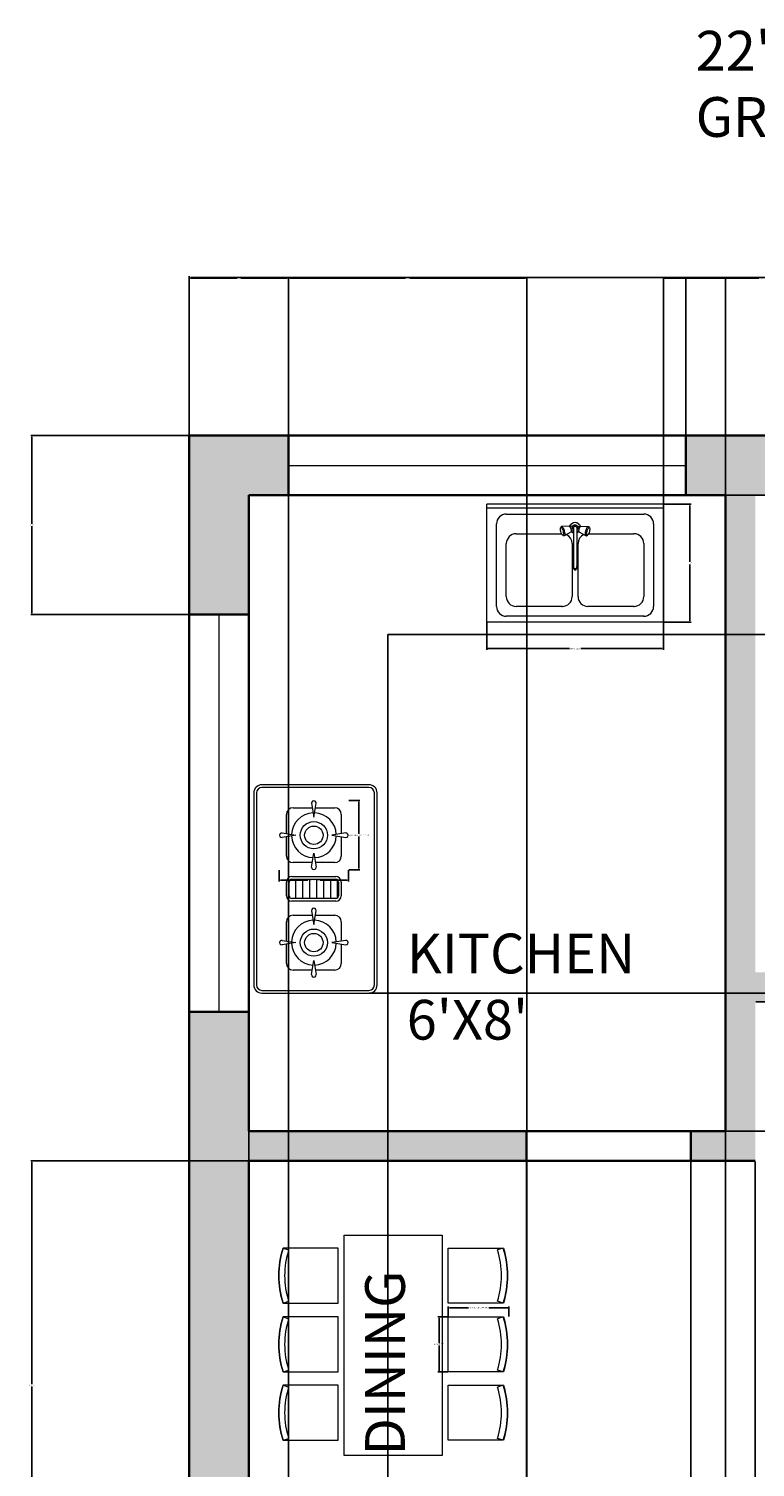
# Model space of a CAD drawing. Units: inches. Extents: x 10 to 332, y -471 to 73.
# Tile 4 of 5: x 10 to 120, y -144 to 73. Entities that reach past the tile are written whole.
import ezdxf

# ---------------------------------------------------------------- set-up
doc = ezdxf.new("R2010")
doc.units = ezdxf.units.IN
doc.header["$MEASUREMENT"] = 0
for name, color, linetype, lineweight in [('A-ANNO-DIMS', 2, 'Continuous', 18), ('A-ANNO-TEXT', 7, 'Continuous', 25), ('A-AREA-IDEN', 7, 'Continuous', 18), ('A-EQPM', 8, 'Continuous', 18), ('A-EQPM-PATT', 8, 'Continuous', 13), ('A-FLOR-CASE', 9, 'Continuous', 25), ('A-FLOR-FIXT', 9, 'Continuous', 18), ('A-FURN', 9, 'Continuous', 18), ('A-GLAZ', 4, 'Continuous', 18), ('A-WALL', 7, 'Continuous', 35), ('A-WALL-PATT', 8, 'Continuous', 13)]:
    doc.layers.add(name, color=color, linetype=linetype, lineweight=lineweight)
doc.styles.get("Standard").update_dxf_attribs({"font": 'arial.ttf'})
doc.dimstyles.get("Standard").update_dxf_attribs({"dimtxt": 0.18, "dimasz": 0.18, "dimexe": 0.18, "dimexo": 0.0625, "dimgap": 0.09, "dimtad": 0, "dimtih": 1, "dimtoh": 1, "dimdec": 0, "dimzin": 0, "dimdsep": 46, "dimlunit": 3, "dimtxsty": 'Standard', "dimcen": 0.09, "dimadec": 0, "dimazin": 0, "dimtfac": 1, "dimtdec": 0, "dimtofl": 0, "dimtmove": 0, "dimatfit": 3, "dimfxl": 1, "dimtolj": 1, "dimtzin": 0, "dimarcsym": 0})

# ---------------------------------------------------------------- blocks, each defined once
blk = doc.blocks.new('М07 600х900')
for p, q in [((0, 600), (-900, 600)), ((-900, 0), (-900, 600)), ((-900, 0), (-900, 600)), ((0, 0), (0, 600)), ((0, 0), (0, 600)), ((0, 580), (-900, 580)), ((-800, 550), (-100, 550)), ((-850, 80), (-850, 500)), ((-750, 450), (-519.1, 450)), ((-524.9, 472.1), (-524.8, 476.7)), ((-524.3, 466.5), (-524.9, 472.1)), ((-524.8, 476.7), (-523.8, 479.9)), ((-523, 460.4), (-524.3, 466.5)), ((-520.9, 485.6), (-523.8, 479.9)), ((-523.8, 479.9), (-522.2, 481.3)), ((-521.1, 454.5), (-523, 460.4)), ((-522.2, 481.3), (-520.1, 480.9)), ((-518.8, 449.4), (-521.1, 454.5)), ((-520.9, 485.6), (-518.9, 487.4)), ((-520.1, 480.9), (-517.7, 478.6)), ((-479.6, 487.6), (-518.9, 487.4)), ((-518.9, 487.4), (-516.3, 486.8)), ((-516.4, 445.5), (-518.8, 449.4)), ((-517.7, 478.6), (-515.3, 474.7)), ((-514, 443.2), (-516.4, 445.5)), ((-516.3, 486.8), (-513.3, 484)), ((-515.3, 474.7), (-513, 469.5)), ((-508.6, 439.7), (-514, 443.2)), ((-511.9, 442.7), (-514, 443.2)), ((-513.3, 484), (-510.2, 479.1)), ((-513, 469.5), (-511.1, 463.6)), ((-510.3, 444.2), (-511.9, 442.7)), ((-511.1, 463.6), (-509.8, 457.6)), ((-509.4, 447.3), (-510.3, 444.2)), ((-510.2, 479.1), (-507.4, 472.6)), ((-509.8, 457.6), (-509.2, 452)), ((-509.2, 452), (-509.4, 447.3)), ((-506, 439.1), (-508.6, 439.7)), ((-507.4, 472.6), (-505, 465.3)), ((-471.8, 458.6), (-506, 439.1)), ((-504, 440.9), (-506, 439.1)), ((-505, 465.3), (-503.4, 457.7)), ((-502.8, 444.9), (-504, 440.9)), ((-503.4, 457.7), (-502.6, 450.7)), ((-502.6, 450.7), (-502.8, 444.9)), ((-479.6, 487.6), (-478, 487.3)), ((-478, 487.3), (-476.2, 485.5)), ((-477, 486.3), (-476.6, 488.7)), ((-476.6, 488.7), (-472.7, 496.5)), ((-461.4, 489.4), (-476.2, 485.4)), ((-476.2, 485.5), (-474.4, 482.6)), ((-474.4, 482.6), (-472.7, 478.7)), ((-472.7, 496.5), (-466.5, 502.7)), ((-472.7, 478.7), (-471.2, 474.3)), ((-470.6, 459.7), (-471.8, 458.6)), ((-471.2, 474.3), (-470.3, 469.8)), ((-469.9, 462.1), (-470.6, 459.7)), ((-470.3, 469.8), (-469.8, 465.6)), ((-466.5, 457.3), (-470.2, 461.1)), ((-469.8, 465.6), (-469.9, 462.1)), ((-458.5, 465.3), (-469.9, 462.2)), ((-466.5, 502.7), (-458.7, 506.6)), ((-458.7, 453.4), (-466.5, 457.3)), ((-465, 480), (-462.1, 488.8)), ((-462.1, 471.2), (-465, 480)), ((-462.1, 488.8), (-454.6, 494.3)), ((-458.5, 468.5), (-462.1, 471.2)), ((-458.7, 506.6), (-450, 508)), ((-458.5, 453.3), (-458.7, 453.4)), ((-458.5, 480), (-456.9, 485)), ((-458.5, 480), (-458.5, 279.9)), ((-456.9, 485), (-452.6, 488.1)), ((-454.6, 494.3), (-445.4, 494.3)), ((-452.6, 488.1), (-447.4, 488.1)), ((-450, 508), (-441.3, 506.6)), ((-447.4, 488.1), (-443.1, 485)), ((-445.4, 494.3), (-437.9, 488.8)), ((-443.1, 485), (-441.5, 480)), ((-441.5, 480), (-441.5, 279.9)), ((-437.9, 471.2), (-441.5, 468.5)), ((-441.5, 465.3), (-430.1, 462.2)), ((-441.3, 453.4), (-441.5, 453.3)), ((-441.3, 506.6), (-433.5, 502.7)), ((-433.5, 457.3), (-441.3, 453.4)), ((-438.6, 489.4), (-423.8, 485.4)), ((-437.9, 488.8), (-435, 480)), ((-435, 480), (-437.9, 471.2)), ((-433.5, 502.7), (-427.3, 496.5)), ((-429.8, 461.1), (-433.5, 457.3)), ((-430.2, 465.6), (-429.7, 469.8)), ((-430.1, 462.1), (-430.2, 465.6)), ((-429.4, 459.7), (-430.1, 462.1)), ((-429.7, 469.8), (-428.8, 474.3)), ((-428.2, 458.6), (-429.4, 459.7)), ((-428.8, 474.3), (-427.3, 478.7)), ((-428.2, 458.6), (-394, 439.1)), ((-427.3, 496.5), (-423.4, 488.7)), ((-427.3, 478.7), (-425.6, 482.6)), ((-425.6, 482.6), (-423.8, 485.5)), ((-423.8, 485.5), (-422, 487.3)), ((-423.4, 488.7), (-423, 486.3)), ((-422, 487.3), (-420.4, 487.6)), ((-420.4, 487.6), (-381.1, 487.4)), ((-397.4, 450.7), (-396.6, 457.7)), ((-397.2, 444.9), (-397.4, 450.7)), ((-396, 440.9), (-397.2, 444.9)), ((-396.6, 457.7), (-395, 465.3)), ((-394, 439.1), (-396, 440.9)), ((-395, 465.3), (-392.6, 472.6)), ((-391.4, 439.7), (-394, 439.1)), ((-392.6, 472.6), (-389.8, 479.1)), ((-391.4, 439.7), (-386, 443.2)), ((-390.8, 452), (-390.2, 457.6)), ((-390.6, 447.3), (-390.8, 452)), ((-389.7, 444.2), (-390.6, 447.3)), ((-390.2, 457.6), (-388.9, 463.6)), ((-389.8, 479.1), (-386.7, 484)), ((-388.1, 442.7), (-389.7, 444.2)), ((-388.9, 463.6), (-387, 469.5)), ((-386, 443.2), (-388.1, 442.7)), ((-387, 469.5), (-384.7, 474.7)), ((-386.7, 484), (-383.7, 486.8)), ((-383.6, 445.5), (-386, 443.2)), ((-384.7, 474.7), (-382.3, 478.6)), ((-383.7, 486.8), (-381.1, 487.4)), ((-381.2, 449.4), (-383.6, 445.5)), ((-382.3, 478.6), (-379.9, 480.9)), ((-378.9, 454.5), (-381.2, 449.4)), ((-381.1, 487.4), (-379.1, 485.6)), ((-380.9, 450), (-150, 450)), ((-379.9, 480.9), (-377.8, 481.3)), ((-379.1, 485.6), (-376.2, 479.9)), ((-377, 460.4), (-378.9, 454.5)), ((-377.8, 481.3), (-376.2, 479.9)), ((-375.7, 466.5), (-377, 460.4)), ((-376.2, 479.9), (-375.2, 476.7)), ((-375.1, 472.1), (-375.7, 466.5)), ((-375.2, 476.7), (-375.1, 472.1)), ((-50, 500), (-50, 80)), ((-800, 130), (-800, 400)), ((-465, 400), (-465, 130)), ((-435, 130), (-435, 400)), ((-100, 400), (-100, 130)), ((-458.5, 285.6), (-460.5, 279.9)), ((-460.5, 279.9), (-458.5, 274.2)), ((-458.5, 279.9), (-456.9, 275.3)), ((-458.5, 274.2), (-456.9, 269.8)), ((-458.5, 274.2), (-453.2, 270.6)), ((-456.9, 275.3), (-452.6, 272.4)), ((-456.9, 269.8), (-452.6, 266.9)), ((-453.2, 270.6), (-446.8, 270.6)), ((-452.6, 272.4), (-447.4, 272.4)), ((-452.6, 266.9), (-447.4, 266.9)), ((-447.4, 272.4), (-443.1, 275.3)), ((-447.4, 266.9), (-443.1, 269.8)), ((-446.8, 270.6), (-441.5, 274.2)), ((-443.1, 275.3), (-441.5, 279.9)), ((-441.5, 274.2), (-443.1, 269.8)), ((-439.5, 279.9), (-441.5, 285.6)), ((-441.5, 274.2), (-439.5, 279.9)), ((-515, 80), (-750, 80)), ((-150, 80), (-385, 80)), ((0, 0), (-900, 0)), ((-100, 30), (-800, 30))]:
    blk.add_line(p, q)
for centre, start, end in [((-800, 500), 90, 180), ((-100, 500), 0, 90), ((-750, 400), 90, 180), ((-515, 400), 0, 65.88741), ((-385, 400), 114.11259, 180), ((-150, 400), 0, 90), ((-800, 80), 180, 270), ((-750, 130), 180, 270), ((-515, 130), 270, 0), ((-385, 130), 180, 270), ((-150, 130), 270, 0), ((-100, 80), 270, 0)]:
    blk.add_arc(centre, 50, start, end)
for p in [(-515, 80), (-150, 80), (-100, 30)]:
    blk.add_point(p)
blk = doc.blocks.new('*D2')
at = {"layer": 'A-ANNO-DIMS', "color": 0, "lineweight": -2, "transparency": 16777216}
for p, q in [((34.37, 12.05), (34.37, 36.05)), ((34.55, 35.87), (157.42, 35.87)), ((301.19, 35.87), (178.31, 35.87)), ((301.37, 12.05), (301.37, 36.05))]:
    blk.add_line(p, q, dxfattribs=at)
at = {"layer": 'A-ANNO-DIMS', "color": 0, "transparency": 16777216}
for points in [[(34.55, 35.9), (34.55, 35.84), (34.37, 35.87)], [(301.19, 35.9), (301.19, 35.84), (301.37, 35.87)]]:
    blk.add_solid(points, dxfattribs=at)
at = {"layer": 'Defpoints', "color": 0, "transparency": 16777216}
for p in [(301.37, 35.87), (34.37, 11.99), (301.37, 11.99)]:
    blk.add_point(p, dxfattribs=at)
at = {"layer": 'A-ANNO-DIMS', "color": 0, "transparency": 16777216, "insert": (167.87, 35.87), "char_height": 6, "attachment_point": 5}
blk.add_mtext('\\A1;22\'-3"', dxfattribs=at)
blk = doc.blocks.new('WIN-60')
for p, q in [((0, 9), (60, 9)), ((0, 4.5), (60, 4.5)), ((60, 0), (0, 0))]:
    blk.add_line(p, q)
blk = doc.blocks.new('CHAIR-DINING')
for p, q in [((8.3, 8.31), (7.42, 8.03)), ((8.3, 0), (7.42, 0.28))]:
    blk.add_line(p, q)
blk.add_lwpolyline([(8.31, 0), (0, 0), (0, 8.31), (8.31, 8.31, -0.153703), (8.31, 0)], format="xyb")
for radius in [12.78, 13.71]:
    blk.add_arc((-4.76, 4.15), radius, 342.3544, 17.6456)
blk = doc.blocks.new('BURNER-GAS')
for p, q in [((2.06, 9.35), (4.98, 9.35)), ((4.87, 10.02), (5.2, 7.92)), ((5.2, 7.92), (5.54, 10.02)), ((5.43, 9.35), (8.35, 9.35)), ((1.06, 5.43), (1.06, 8.35)), ((9.34, 8.35), (9.34, 5.43)), ((0.39, 5.54), (2.49, 5.2)), ((2.49, 5.2), (0.39, 4.87)), ((1.06, 2.06), (1.06, 4.98)), ((10.02, 5.54), (7.92, 5.2)), ((7.92, 5.2), (10.02, 4.87)), ((9.34, 4.98), (9.34, 2.06)), ((4.87, 0.39), (5.2, 2.49)), ((5.2, 2.49), (5.54, 0.39)), ((4.98, 1.06), (2.06, 1.06)), ((8.35, 1.06), (5.43, 1.06))]:
    blk.add_line(p, q)
for radius in [2.05, 1.39]:
    blk.add_circle((5.2, 5.2), radius)
for centre, radius, start, end in [((2.06, 8.35), 0.994, 90, 180), ((5.2, 10.07), 0.335, 351.0363, 188.9637), ((8.35, 8.35), 0.994, 0, 90), ((5.2, 5.2), 3.38, 91.7678, 178.2322), ((5.2, 5.2), 3.38, 1.7678, 88.2322), ((0.34, 5.2), 0.335, 81.0363, 278.9637), ((5.2, 5.2), 3.38, 181.7678, 268.2322), ((5.2, 5.2), 3.38, 271.7678, 358.2322), ((10.07, 5.2), 0.335, 261.0363, 98.9637), ((2.06, 2.06), 0.994, 180, 270), ((5.2, 0.34), 0.335, 171.0363, 8.9637), ((8.35, 2.06), 0.994, 270, 0)]:
    blk.add_arc(centre, radius, start, end)
blk = doc.blocks.new('*D14')
at = {"layer": 'A-ANNO-DIMS', "color": 0, "lineweight": -2, "transparency": 16777216}
for p, q in [((73.51, -120.97), (73.51, -119.48)), ((73.69, -119.66), (76.55, -119.66)), ((82.49, -119.66), (79.62, -119.66)), ((82.67, -120.97), (82.67, -119.48))]:
    blk.add_line(p, q, dxfattribs=at)
at = {"layer": 'A-ANNO-DIMS', "color": 0, "transparency": 16777216}
for points in [[(73.69, -119.63), (73.69, -119.69), (73.51, -119.66)], [(82.49, -119.63), (82.49, -119.69), (82.67, -119.66)]]:
    blk.add_solid(points, dxfattribs=at)
at = {"layer": 'Defpoints', "color": 0, "transparency": 16777216}
for p in [(73.51, -121.04), (82.67, -119.66), (82.67, -121.04)]:
    blk.add_point(p, dxfattribs=at)
at = {"layer": 'A-ANNO-DIMS', "color": 0, "transparency": 16777216, "insert": (78.09, -119.66), "char_height": 0.18, "attachment_point": 5}
blk.add_mtext('\\A1;DINING CHAIR 0\'-9" TYP.', dxfattribs=at)
blk = doc.blocks.new('*D15')
at = {"layer": 'A-ANNO-DIMS', "color": 0, "lineweight": -2, "transparency": 16777216}
for p, q in [((73.44, -121.04), (71.95, -121.04)), ((72.13, -121.22), (72.13, -125.01)), ((72.13, -129.17), (72.13, -125.37)), ((73.44, -129.35), (71.95, -129.35))]:
    blk.add_line(p, q, dxfattribs=at)
at = {"layer": 'A-ANNO-DIMS', "color": 0, "transparency": 16777216}
for points in [[(72.1, -121.22), (72.16, -121.22), (72.13, -121.04)], [(72.1, -129.17), (72.16, -129.17), (72.13, -129.35)]]:
    blk.add_solid(points, dxfattribs=at)
at = {"layer": 'Defpoints', "color": 0, "transparency": 16777216}
for p in [(72.13, -121.04), (73.51, -121.04), (73.51, -129.35)]:
    blk.add_point(p, dxfattribs=at)
at = {"layer": 'A-ANNO-DIMS', "color": 0, "transparency": 16777216, "insert": (72.13, -125.19), "char_height": 0.18, "attachment_point": 5}
blk.add_mtext('\\A1;0\'-8 1/2" TYP.', dxfattribs=at)
blk = doc.blocks.new('*D26')
at = {"layer": 'A-ANNO-DIMS', "color": 0, "lineweight": -2, "transparency": 16777216}
for p, q in [((58.49, -43.11), (60.17, -43.11)), ((59.99, -43.29), (59.99, -48.15)), ((59.99, -53.38), (59.99, -48.52)), ((58.49, -53.56), (60.17, -53.56))]:
    blk.add_line(p, q, dxfattribs=at)
at = {"layer": 'A-ANNO-DIMS', "color": 0, "transparency": 16777216}
for points in [[(59.96, -43.29), (60.02, -43.29), (59.99, -43.11)], [(59.96, -53.38), (60.02, -53.38), (59.99, -53.56)]]:
    blk.add_solid(points, dxfattribs=at)
at = {"layer": 'Defpoints', "color": 0, "transparency": 16777216}
for p in [(58.42, -43.11), (59.99, -43.11), (58.42, -53.56)]:
    blk.add_point(p, dxfattribs=at)
at = {"layer": 'A-ANNO-DIMS', "color": 0, "transparency": 16777216, "insert": (59.99, -48.33), "char_height": 0.18, "attachment_point": 5}
blk.add_mtext('\\A1;GAS BURNER 0\'-10 1/2" TYP.', dxfattribs=at)
blk = doc.blocks.new('*D27')
at = {"layer": 'A-ANNO-DIMS', "color": 0, "lineweight": -2, "transparency": 16777216}
for p, q in [((47.98, -53.62), (47.98, -55.3)), ((58.42, -53.62), (58.42, -55.3)), ((48.16, -55.12), (52.28, -55.12)), ((58.24, -55.12), (54.12, -55.12))]:
    blk.add_line(p, q, dxfattribs=at)
at = {"layer": 'A-ANNO-DIMS', "color": 0, "transparency": 16777216}
for points in [[(48.16, -55.09), (48.16, -55.15), (47.98, -55.12)], [(58.24, -55.09), (58.24, -55.15), (58.42, -55.12)]]:
    blk.add_solid(points, dxfattribs=at)
at = {"layer": 'Defpoints', "color": 0, "transparency": 16777216}
for p in [(47.98, -53.56), (58.42, -53.56), (58.42, -55.12)]:
    blk.add_point(p, dxfattribs=at)
at = {"layer": 'A-ANNO-DIMS', "color": 0, "transparency": 16777216, "insert": (53.2, -55.12), "char_height": 0.18, "attachment_point": 5}
blk.add_mtext('\\A1;0\'-10 1/2" TYP.', dxfattribs=at)
blk = doc.blocks.new('*D28')
at = {"layer": 'A-ANNO-DIMS', "color": 0, "lineweight": -2, "transparency": 16777216}
for p, q in [((79.31, -16.23), (79.31, -20.35)), ((106, -16.23), (106, -20.35)), ((79.49, -20.17), (91.79, -20.17)), ((105.82, -20.17), (93.52, -20.17))]:
    blk.add_line(p, q, dxfattribs=at)
at = {"layer": 'A-ANNO-DIMS', "color": 0, "transparency": 16777216}
for points in [[(79.49, -20.14), (79.49, -20.2), (79.31, -20.17)], [(105.82, -20.14), (105.82, -20.2), (106, -20.17)]]:
    blk.add_solid(points, dxfattribs=at)
at = {"layer": 'Defpoints', "color": 0, "transparency": 16777216}
for p in [(79.31, -16.17), (106, -16.17), (106, -20.17)]:
    blk.add_point(p, dxfattribs=at)
at = {"layer": 'A-ANNO-DIMS', "color": 0, "transparency": 16777216, "insert": (92.65, -20.17), "char_height": 0.18, "attachment_point": 5}
blk.add_mtext('\\A1;SINK 2\'-2 1/2"', dxfattribs=at)
blk = doc.blocks.new('*D29')
at = {"layer": 'A-ANNO-DIMS', "color": 0, "lineweight": -2, "transparency": 16777216}
for p, q in [((106.06, 1.63), (110.19, 1.63)), ((110.01, 1.45), (110.01, -7.09)), ((110.01, -15.99), (110.01, -7.45)), ((106.06, -16.17), (110.19, -16.17))]:
    blk.add_line(p, q, dxfattribs=at)
at = {"layer": 'A-ANNO-DIMS', "color": 0, "transparency": 16777216}
for points in [[(109.98, 1.45), (110.04, 1.45), (110.01, 1.63)], [(109.98, -15.99), (110.04, -15.99), (110.01, -16.17)]]:
    blk.add_solid(points, dxfattribs=at)
at = {"layer": 'Defpoints', "color": 0, "transparency": 16777216}
for p in [(106, 1.63), (110.01, 1.63), (106, -16.17)]:
    blk.add_point(p, dxfattribs=at)
at = {"layer": 'A-ANNO-DIMS', "color": 0, "transparency": 16777216, "insert": (110.01, -7.27), "char_height": 0.18, "attachment_point": 5}
blk.add_mtext('\\A1;1\'-6"', dxfattribs=at)
blk = doc.blocks.new('*D30')
at = {"layer": 'A-ANNO-DIMS', "color": 0, "lineweight": -2, "transparency": 16777216}
for p, q in [((167.87, -93.08), (167.87, -470.94)), ((43.37, -97.58), (43.37, -470.94)), ((43.55, -470.76), (105.02, -470.76)), ((167.69, -470.76), (106.22, -470.76))]:
    blk.add_line(p, q, dxfattribs=at)
at = {"layer": 'A-ANNO-DIMS', "color": 0, "transparency": 16777216}
for points in [[(43.55, -470.73), (43.55, -470.79), (43.37, -470.76)], [(167.69, -470.73), (167.69, -470.79), (167.87, -470.76)]]:
    blk.add_solid(points, dxfattribs=at)
at = {"layer": 'Defpoints', "color": 0, "transparency": 16777216}
for p in [(167.87, -93.01), (43.37, -97.51), (167.87, -470.76)]:
    blk.add_point(p, dxfattribs=at)
at = {"layer": 'A-ANNO-DIMS', "color": 0, "transparency": 16777216, "insert": (105.62, -470.76), "char_height": 0.18, "attachment_point": 5}
blk.add_mtext('\\A1;10\'-4 1/2"', dxfattribs=at)
blk = doc.blocks.new('*D37')
at = {"layer": 'A-ANNO-DIMS', "color": 0, "lineweight": -2, "transparency": 16777216}
for p, q in [((34.37, 12.05), (34.37, 35.92)), ((34.55, 35.74), (41.55, 35.74)), ((49.19, 35.74), (42.19, 35.74)), ((49.37, 12.05), (49.37, 35.92))]:
    blk.add_line(p, q, dxfattribs=at)
at = {"layer": 'A-ANNO-DIMS', "color": 0, "transparency": 16777216}
for points in [[(34.55, 35.77), (34.55, 35.71), (34.37, 35.74)], [(49.19, 35.77), (49.19, 35.71), (49.37, 35.74)]]:
    blk.add_solid(points, dxfattribs=at)
at = {"layer": 'Defpoints', "color": 0, "transparency": 16777216}
for p in [(49.37, 35.74), (34.37, 11.99), (49.37, 11.99)]:
    blk.add_point(p, dxfattribs=at)
at = {"layer": 'A-ANNO-DIMS', "color": 0, "transparency": 16777216, "insert": (41.87, 35.74), "char_height": 0.18, "attachment_point": 5}
blk.add_mtext('\\A1;1\'-3"', dxfattribs=at)
blk = doc.blocks.new('*D39')
at = {"layer": 'A-ANNO-DIMS', "color": 0, "lineweight": -2, "transparency": 16777216}
for p, q in [((34.3, 11.99), (10.44, 11.99)), ((10.62, 11.81), (10.62, -1.33)), ((10.62, -14.83), (10.62, -1.7)), ((34.3, -15.01), (10.44, -15.01))]:
    blk.add_line(p, q, dxfattribs=at)
at = {"layer": 'A-ANNO-DIMS', "color": 0, "transparency": 16777216}
for points in [[(10.59, 11.81), (10.65, 11.81), (10.62, 11.99)], [(10.59, -14.83), (10.65, -14.83), (10.62, -15.01)]]:
    blk.add_solid(points, dxfattribs=at)
at = {"layer": 'Defpoints', "color": 0, "transparency": 16777216}
for p in [(34.37, 11.99), (10.62, -15.01), (34.37, -15.01)]:
    blk.add_point(p, dxfattribs=at)
at = {"layer": 'A-ANNO-DIMS', "color": 0, "transparency": 16777216, "insert": (10.62, -1.51), "char_height": 0.18, "attachment_point": 5}
blk.add_mtext('\\A1;2\'-3"', dxfattribs=at)
blk = doc.blocks.new('*D40')
at = {"layer": 'A-ANNO-DIMS', "color": 0, "lineweight": -2, "transparency": 16777216}
for p, q in [((43.3, -97.51), (10.44, -97.51)), ((10.62, -97.69), (10.62, -131.18)), ((10.62, -165.02), (10.62, -131.54)), ((43.3, -165.2), (10.44, -165.2))]:
    blk.add_line(p, q, dxfattribs=at)
at = {"layer": 'A-ANNO-DIMS', "color": 0, "transparency": 16777216}
for points in [[(10.59, -97.69), (10.65, -97.69), (10.62, -97.51)], [(10.59, -165.02), (10.65, -165.02), (10.62, -165.2)]]:
    blk.add_solid(points, dxfattribs=at)
at = {"layer": 'Defpoints', "color": 0, "transparency": 16777216}
for p in [(43.37, -97.51), (10.62, -165.2), (43.37, -165.2)]:
    blk.add_point(p, dxfattribs=at)
at = {"layer": 'A-ANNO-DIMS', "color": 0, "transparency": 16777216, "insert": (10.62, -131.36), "char_height": 0.18, "attachment_point": 5}
blk.add_mtext('\\A1;5\'-7 1/2"', dxfattribs=at)
blk = doc.blocks.new('*D46')
at = {"layer": 'A-ANNO-DIMS', "color": 0, "lineweight": -2, "transparency": 16777216}
for p, q in [((43.37, -93.08), (43.37, -470.94)), ((64.36, -93.08), (64.36, -470.94)), ((43.55, -470.76), (53.54, -470.76)), ((64.18, -470.76), (54.18, -470.76))]:
    blk.add_line(p, q, dxfattribs=at)
at = {"layer": 'A-ANNO-DIMS', "color": 0, "transparency": 16777216}
for points in [[(43.55, -470.73), (43.55, -470.79), (43.37, -470.76)], [(64.18, -470.73), (64.18, -470.79), (64.36, -470.76)]]:
    blk.add_solid(points, dxfattribs=at)
at = {"layer": 'Defpoints', "color": 0, "transparency": 16777216}
for p in [(43.37, -93.01), (64.36, -93.01), (64.36, -470.76)]:
    blk.add_point(p, dxfattribs=at)
at = {"layer": 'A-ANNO-DIMS', "color": 0, "transparency": 16777216, "insert": (53.86, -470.76), "char_height": 0.18, "attachment_point": 5}
blk.add_mtext('\\A1;1\'-9"', dxfattribs=at)
blk = doc.blocks.new('*D47')
at = {"layer": 'A-ANNO-DIMS', "color": 0, "lineweight": -2, "transparency": 16777216}
for p, q in [((115.43, 2.99), (325.3, 2.99)), ((325.12, 2.81), (325.12, -7.34)), ((325.12, -17.85), (325.12, -7.7)), ((115.43, -18.03), (325.3, -18.03))]:
    blk.add_line(p, q, dxfattribs=at)
at = {"layer": 'A-ANNO-DIMS', "color": 0, "transparency": 16777216}
for points in [[(325.09, 2.81), (325.15, 2.81), (325.12, 2.99)], [(325.09, -17.85), (325.15, -17.85), (325.12, -18.03)]]:
    blk.add_solid(points, dxfattribs=at)
at = {"layer": 'Defpoints', "color": 0, "transparency": 16777216}
for p in [(115.37, 2.99), (115.37, -18.03), (325.12, -18.03)]:
    blk.add_point(p, dxfattribs=at)
at = {"layer": 'A-ANNO-DIMS', "color": 0, "transparency": 16777216, "insert": (325.12, -7.52), "char_height": 0.18, "attachment_point": 5}
blk.add_mtext('\\A1;1\'-9"', dxfattribs=at)
blk = doc.blocks.new('*D48')
at = {"layer": 'A-ANNO-DIMS', "color": 0, "lineweight": -2, "transparency": 16777216}
for p, q in [((85.3, -93.08), (85.3, -470.94)), ((110.16, -93.08), (110.16, -470.94)), ((85.48, -470.76), (97.4, -470.76)), ((109.98, -470.76), (98.06, -470.76))]:
    blk.add_line(p, q, dxfattribs=at)
at = {"layer": 'A-ANNO-DIMS', "color": 0, "transparency": 16777216}
for points in [[(85.48, -470.73), (85.48, -470.79), (85.3, -470.76)], [(109.98, -470.73), (109.98, -470.79), (110.16, -470.76)]]:
    blk.add_solid(points, dxfattribs=at)
at = {"layer": 'Defpoints', "color": 0, "transparency": 16777216}
for p in [(85.3, -93.01), (110.16, -93.01), (110.16, -470.76)]:
    blk.add_point(p, dxfattribs=at)
at = {"layer": 'A-ANNO-DIMS', "color": 0, "transparency": 16777216, "insert": (97.73, -470.76), "char_height": 0.18, "attachment_point": 5}
blk.add_mtext('\\A1;2\'-1"', dxfattribs=at)
blk = doc.blocks.new('*D49')
at = {"layer": 'A-ANNO-DIMS', "color": 0, "lineweight": -2, "transparency": 16777216}
for p, q in [((119.93, -73.51), (325.3, -73.51)), ((325.12, -73.69), (325.12, -83.08)), ((325.12, -92.83), (325.12, -83.45)), ((119.93, -93.01), (325.3, -93.01))]:
    blk.add_line(p, q, dxfattribs=at)
at = {"layer": 'A-ANNO-DIMS', "color": 0, "transparency": 16777216}
for points in [[(325.09, -73.69), (325.15, -73.69), (325.12, -73.51)], [(325.09, -92.83), (325.15, -92.83), (325.12, -93.01)]]:
    blk.add_solid(points, dxfattribs=at)
at = {"layer": 'Defpoints', "color": 0, "transparency": 16777216}
for p in [(119.87, -73.51), (119.87, -93.01), (325.12, -93.01)]:
    blk.add_point(p, dxfattribs=at)
at = {"layer": 'A-ANNO-DIMS', "color": 0, "transparency": 16777216, "insert": (325.12, -83.26), "char_height": 0.18, "attachment_point": 5}
blk.add_mtext('\\A1;1\'-7 1/2"', dxfattribs=at)
blk = doc.blocks.new('*D50')
at = {"layer": 'A-ANNO-DIMS', "color": 0, "lineweight": -2, "transparency": 16777216}
for p, q in [((115.37, -93.08), (115.37, -470.94)), ((119.87, -97.58), (119.87, -470.94)), ((115.55, -470.76), (117.08, -470.76)), ((119.69, -470.76), (118.16, -470.76))]:
    blk.add_line(p, q, dxfattribs=at)
at = {"layer": 'A-ANNO-DIMS', "color": 0, "transparency": 16777216}
for points in [[(115.55, -470.73), (115.55, -470.79), (115.37, -470.76)], [(119.69, -470.73), (119.69, -470.79), (119.87, -470.76)]]:
    blk.add_solid(points, dxfattribs=at)
at = {"layer": 'Defpoints', "color": 0, "transparency": 16777216}
for p in [(115.37, -93.01), (119.87, -97.51), (119.87, -470.76)]:
    blk.add_point(p, dxfattribs=at)
at = {"layer": 'A-ANNO-DIMS', "color": 0, "transparency": 16777216, "insert": (117.62, -470.76), "char_height": 0.18, "attachment_point": 5}
blk.add_mtext('\\A1;0\'-4 1/2"', dxfattribs=at)
blk = doc.blocks.new('*D52')
at = {"layer": 'A-ANNO-DIMS', "color": 0, "lineweight": -2, "transparency": 16777216}
for p, q in [((109.37, 12.05), (109.37, 35.92)), ((109.55, 35.74), (120.41, 35.74)), ((132.48, 35.74), (121.61, 35.74)), ((132.66, 12.05), (132.66, 35.92))]:
    blk.add_line(p, q, dxfattribs=at)
at = {"layer": 'A-ANNO-DIMS', "color": 0, "transparency": 16777216}
for points in [[(109.55, 35.77), (109.55, 35.71), (109.37, 35.74)], [(132.48, 35.77), (132.48, 35.71), (132.66, 35.74)]]:
    blk.add_solid(points, dxfattribs=at)
at = {"layer": 'Defpoints', "color": 0, "transparency": 16777216}
for p in [(132.66, 35.74), (109.37, 11.99), (132.66, 11.99)]:
    blk.add_point(p, dxfattribs=at)
at = {"layer": 'A-ANNO-DIMS', "color": 0, "transparency": 16777216, "insert": (121.01, 35.74), "char_height": 0.18, "attachment_point": 5}
blk.add_mtext('\\A1;1\'-11 1/2"', dxfattribs=at)
blk = doc.blocks.new('*D54')
at = {"layer": 'A-ANNO-DIMS', "color": 0, "lineweight": -2, "transparency": 16777216}
for p, q in [((49.37, -418.45), (49.37, 35.92)), ((49.55, 35.74), (67.04, 35.74)), ((85.19, 35.74), (67.7, 35.74)), ((85.37, -418.45), (85.37, 35.92))]:
    blk.add_line(p, q, dxfattribs=at)
at = {"layer": 'A-ANNO-DIMS', "color": 0, "transparency": 16777216}
for points in [[(49.55, 35.77), (49.55, 35.71), (49.37, 35.74)], [(85.19, 35.77), (85.19, 35.71), (85.37, 35.74)]]:
    blk.add_solid(points, dxfattribs=at)
at = {"layer": 'Defpoints', "color": 0, "transparency": 16777216}
for p in [(85.37, 35.74), (49.37, -418.51), (85.37, -418.51)]:
    blk.add_point(p, dxfattribs=at)
at = {"layer": 'A-ANNO-DIMS', "color": 0, "transparency": 16777216, "insert": (67.37, 35.74), "char_height": 0.18, "attachment_point": 5}
blk.add_mtext('\\A1;3\'-0"', dxfattribs=at)
blk = doc.blocks.new('*D55')
at = {"layer": 'A-ANNO-DIMS', "color": 0, "lineweight": -2, "transparency": 16777216}
for p, q in [((106, -16.11), (106, 35.92)), ((106.18, 35.74), (110.15, 35.74)), ((115.19, 35.74), (111.22, 35.74)), ((115.37, -17.96), (115.37, 35.92))]:
    blk.add_line(p, q, dxfattribs=at)
at = {"layer": 'A-ANNO-DIMS', "color": 0, "transparency": 16777216}
for points in [[(106.18, 35.77), (106.18, 35.71), (106, 35.74)], [(115.19, 35.77), (115.19, 35.71), (115.37, 35.74)]]:
    blk.add_solid(points, dxfattribs=at)
at = {"layer": 'Defpoints', "color": 0, "transparency": 16777216}
for p in [(115.37, 35.74), (106, -16.17), (115.37, -18.03)]:
    blk.add_point(p, dxfattribs=at)
at = {"layer": 'A-ANNO-DIMS', "color": 0, "transparency": 16777216, "insert": (110.68, 35.74), "char_height": 0.18, "attachment_point": 5}
blk.add_mtext('\\A1;0\'-9 1/2"', dxfattribs=at)
blk = doc.blocks.new('*D56')
at = {"layer": 'A-ANNO-DIMS', "color": 0, "lineweight": -2, "transparency": 16777216}
for p, q in [((61.57, -72.18), (325.3, -72.18)), ((325.12, -72.36), (325.12, -82.41)), ((325.12, -92.83), (325.12, -82.78)), ((64.42, -93.01), (325.3, -93.01))]:
    blk.add_line(p, q, dxfattribs=at)
at = {"layer": 'A-ANNO-DIMS', "color": 0, "transparency": 16777216}
for points in [[(325.09, -72.36), (325.15, -72.36), (325.12, -72.18)], [(325.09, -92.83), (325.15, -92.83), (325.12, -93.01)]]:
    blk.add_solid(points, dxfattribs=at)
at = {"layer": 'Defpoints', "color": 0, "transparency": 16777216}
for p in [(61.51, -72.18), (325.12, -72.18), (64.36, -93.01)]:
    blk.add_point(p, dxfattribs=at)
at = {"layer": 'A-ANNO-DIMS', "color": 0, "transparency": 16777216, "insert": (325.12, -82.6), "char_height": 0.18, "attachment_point": 5}
blk.add_mtext('\\A1;1\'-9"', dxfattribs=at)

msp = doc.modelspace()

# ---------------------------------------------------------------- hatches: boundary and pattern name
at = {"layer": 'A-EQPM-PATT'}
h = msp.add_hatch(dxfattribs=at)
h.set_pattern_fill('ANSI31', color=256, scale=8.414, angle=45, style=0)
h.paths.add_polyline_path([(56.93, -55.4), (56.93, -55.36), (56.92, -55.32), (56.91, -55.28), (56.9, -55.24), (56.88, -55.21), (56.86, -55.17), (56.83, -55.14), (56.81, -55.11), (56.78, -55.08), (56.74, -55.06), (56.71, -55.04), (56.67, -55.02), (56.63, -55.01), (56.6, -55), (56.56, -54.99), (56.51, -54.99), (49.89, -54.99), (49.85, -54.99), (49.81, -55), (49.77, -55.01), (49.73, -55.02), (49.69, -55.04), (49.66, -55.06), (49.63, -55.08), (49.6, -55.11), (49.57, -55.14), (49.55, -55.17), (49.52, -55.21), (49.51, -55.24), (49.49, -55.28), (49.48, -55.32), (49.48, -55.36), (49.48, -55.4), (49.48, -57.48), (49.48, -57.52), (49.48, -57.56), (49.49, -57.6), (49.51, -57.64), (49.52, -57.68), (49.55, -57.71), (49.57, -57.75), (49.6, -57.78), (49.63, -57.8), (49.66, -57.83), (49.69, -57.85), (49.73, -57.87), (49.77, -57.88), (49.81, -57.89), (49.85, -57.89), (49.89, -57.9), (56.51, -57.9), (56.56, -57.89), (56.6, -57.89), (56.63, -57.88), (56.67, -57.87), (56.71, -57.85), (56.74, -57.83), (56.78, -57.8), (56.81, -57.78), (56.83, -57.75), (56.86, -57.71), (56.88, -57.68), (56.9, -57.64), (56.91, -57.6), (56.92, -57.56), (56.93, -57.52), (56.93, -57.48)])
at = {"layer": 'A-WALL-PATT'}
h = msp.add_hatch(color=256, dxfattribs=at)
h.dxf.hatch_style = 1
h.paths.add_polyline_path([(132.66, 11.99), (109.37, 11.99), (109.37, 2.98), (115.37, 2.98), (115.37, -93.01), (110.16, -93.01), (110.16, -97.51), (119.87, -97.51), (119.87, -73.51), (167.87, -73.51), (167.87, -107.01), (170.12, -107.01), (172.37, -107.01), (172.37, -63.01), (167.87, -63.01), (167.87, -69.01), (119.87, -69.01), (119.87, 2.98), (132.66, 2.98)])
h.paths.add_polyline_path([(202.37, 11.99), (152.96, 11.99), (152.96, 2.98), (167.87, 2.98), (167.87, -35.01), (170.12, -35.01), (172.37, -35.01), (172.37, 2.98), (202.37, 2.98)])
h.paths.add_polyline_path([(49.37, 11.99), (34.37, 11.99), (34.37, -15.01), (43.37, -15.01), (43.37, 2.98), (49.37, 2.98)])
h.paths.add_polyline_path([(301.37, 11.99), (262.37, 11.99), (262.37, 2.98), (292.37, 2.98), (292.37, -39.01), (301.37, -39.01)])
h.paths.add_polyline_path([(85.3, -93.01), (43.37, -93.01), (43.37, -75.01), (34.37, -75.01), (34.37, -165.2), (43.37, -165.2), (43.37, -97.51), (85.3, -97.51)])
h.paths.add_polyline_path([(43.37, -225.2), (34.37, -225.2), (34.37, -427.51), (49.37, -427.51), (49.37, -418.51), (43.37, -418.51), (43.37, -346.51), (49.4, -346.51), (49.4, -342.01), (43.37, -342.01)])
h.paths.add_polyline_path([(105.62, -342.01), (86.21, -342.01), (86.21, -346.51), (91.37, -346.51), (91.37, -418.51), (85.37, -418.51), (85.37, -427.51), (101.87, -427.51), (101.87, -418.51), (95.87, -418.51), (95.87, -346.51), (105.62, -346.51)])
h.paths.add_polyline_path([(301.37, -312.01), (292.37, -312.01), (292.37, -342.01), (172.37, -342.01), (172.37, -179.51), (170.12, -179.51), (167.87, -179.51), (167.87, -342.01), (158.84, -342.01), (158.84, -346.51), (292.37, -346.51), (292.37, -352.51), (301.37, -352.51)])
h.paths.add_polyline_path([(301.37, -412.51), (292.37, -412.51), (292.37, -418.51), (153.87, -418.51), (153.87, -423.01), (153.87, -427.51), (301.37, -427.51)])
h.paths.add_polyline_path([(301.37, -99.01), (292.37, -99.01), (292.37, -141.01), (172.37, -141.01), (172.37, -135.01), (167.87, -135.01), (167.87, -151.51), (172.37, -151.51), (172.37, -145.51), (292.37, -145.51), (292.37, -165.79), (301.37, -165.79)])

# ---------------------------------------------------------------- linework, layer by layer
at = {"layer": 'A-EQPM'}
for p, q in [((61.51, -40.71), (45.36, -40.71)), ((61.51, -41.12), (45.36, -41.12)), ((44.12, -41.95), (44.12, -70.93)), ((44.53, -41.95), (44.53, -70.93)), ((62.34, -70.93), (62.34, -41.95)), ((62.75, -70.93), (62.75, -41.95)), ((49.06, -57.48), (49.06, -55.4)), ((49.48, -57.48), (49.48, -55.4)), ((49.89, -54.57), (56.51, -54.57)), ((49.89, -54.99), (56.51, -54.99)), ((56.93, -55.4), (56.93, -57.48)), ((57.34, -55.4), (57.34, -57.48)), ((56.51, -57.9), (49.89, -57.9)), ((56.51, -58.31), (49.89, -58.31)), ((45.36, -71.76), (61.51, -71.76)), ((45.36, -72.18), (61.51, -72.18))]:
    msp.add_line(p, q, dxfattribs=at)
for centre, radius, start, end in [((45.36, -41.95), 1.24, 90, 180), ((45.36, -41.95), 0.828, 90, 180), ((61.51, -41.95), 1.24, 0, 90), ((61.51, -41.95), 0.828, 0, 90), ((49.89, -55.4), 0.828, 90, 180), ((49.89, -55.4), 0.414, 90, 180), ((56.51, -55.4), 0.828, 0, 90), ((56.51, -55.4), 0.414, 0, 90), ((49.89, -57.48), 0.828, 180, 270), ((49.89, -57.48), 0.414, 180, 270), ((56.51, -57.48), 0.414, 270, 0), ((56.51, -57.48), 0.828, 270, 0), ((45.36, -70.93), 1.24, 180, 270), ((45.36, -70.93), 0.828, 180, 270), ((61.51, -70.93), 0.828, 270, 0), ((61.51, -70.93), 1.24, 270, 0)]:
    msp.add_arc(centre, radius, start, end, dxfattribs=at)
at = {"layer": 'A-FLOR-CASE'}
for p, q in [((115.37, -18.03), (64.36, -18.03)), ((64.36, -18.03), (64.36, -93.01))]:
    msp.add_line(p, q, dxfattribs=at)
at = {"layer": 'A-FURN'}
msp.add_lwpolyline([(57.79, -108.72), (72.57, -108.72), (72.57, -141.96), (57.79, -141.96)], close=True, dxfattribs=at)
at = {"layer": 'A-WALL'}
for p, q in [((34.37, 11.99), (34.37, -427.51)), ((34.37, 11.99), (301.37, 11.99)), ((49.37, 2.98), (49.37, 11.99)), ((109.37, 11.99), (109.37, 2.98)), ((43.37, 2.98), (115.37, 2.98)), ((43.37, 2.98), (43.37, -93.01)), ((115.37, 2.98), (115.37, -93.01)), ((34.37, -15.01), (43.37, -15.01)), ((43.37, -75.01), (34.37, -75.01)), ((43.37, -93.01), (115.37, -93.01)), ((85.3, -93.01), (85.3, -97.51)), ((110.16, -93.01), (110.16, -97.51)), ((43.37, -97.51), (119.87, -97.51)), ((43.37, -97.51), (43.37, -342.01))]:
    msp.add_line(p, q, dxfattribs=at)

# ---------------------------------------------------------------- block references
at = {"layer": 'A-EQPM'}
for p in [(48, -53.54), (48, -69.75)]:
    msp.add_blockref('BURNER-GAS', p, dxfattribs=at)
at = {"layer": 'A-FLOR-FIXT', "xscale": 0.0296607722559947, "yscale": 0.0296607722559947, "zscale": 0.0296607722559947}
msp.add_blockref('М07 600х900', (106, -16.17), dxfattribs=at)
at = {"layer": 'A-FURN', "extrusion": (0, 0, -1), "zscale": -1}
for p in [(-56.86, -118.96), (-56.86, -129.35), (-56.86, -139.67)]:
    msp.add_blockref('CHAIR-DINING', p, dxfattribs=at)
at = {"layer": 'A-FURN'}
for p in [(73.51, -118.96), (73.51, -129.35), (73.51, -139.67)]:
    msp.add_blockref('CHAIR-DINING', p, dxfattribs=at)
at = {"layer": 'A-GLAZ'}
msp.add_blockref('WIN-60', (49.37, 2.98), dxfattribs=at)
at = {"layer": 'A-GLAZ', "rotation": 270}
msp.add_blockref('WIN-60', (34.37, -15.01), dxfattribs=at)

# ---------------------------------------------------------------- texts
at = {"layer": 'A-ANNO-TEXT', "insert": (110.87, 73.08), "char_height": 6, "attachment_point": 1}
msp.add_mtext("22'6X34'11 EAST FACING HOUSE PLAN\\PGROUND FLOOR BIKRAM BAURI", dxfattribs=at)
at = {"layer": 'A-AREA-IDEN', "insert": (67.23, -63.19), "char_height": 6, "attachment_point": 1}
msp.add_mtext("KITCHEN\\P6'X8'", dxfattribs=at)
at = {"layer": 'A-AREA-IDEN', "insert": (60.95, -141.96), "char_height": 6, "attachment_point": 1, "rotation": 90}
msp.add_mtext('DINING', dxfattribs=at)

# ---------------------------------------------------------------- dimensions: what is measured, and where the dimension line sits
at = {"layer": 'A-ANNO-DIMS'}
for base, p1, p2, override, picture, middle in [((301.37, 35.87), (34.37, 11.99), (301.37, 11.99), {"dimtxt": 6, "dimclrd": 0, "dimclre": 0, "dimclrt": 0}, '*D2', (167.87, 35.87)), ((49.37, 35.74), (34.37, 11.99), (49.37, 11.99), {"dimdec": 1, "dimlfac": 1, "dimrnd": 0, "dimzin": 1, "dimdsep": 46, "dimlunit": 4, "dimfrac": 2}, '*D37', (41.87, 35.74)), ((85.37, 35.74), (49.37, -418.51), (85.37, -418.51), {"dimdec": 1, "dimlfac": 1, "dimrnd": 0, "dimzin": 1, "dimdsep": 46, "dimlunit": 4, "dimfrac": 2}, '*D54', (67.37, 35.74)), ((115.37, 35.74), (106, -16.17), (115.37, -18.03), {"dimdec": 1, "dimlfac": 1, "dimrnd": 0, "dimzin": 1, "dimdsep": 46, "dimlunit": 4, "dimfrac": 2}, '*D55', (110.68, 35.74)), ((132.66, 35.74), (109.37, 11.99), (132.66, 11.99), {"dimdec": 1, "dimlfac": 1, "dimrnd": 0, "dimzin": 1, "dimdsep": 46, "dimlunit": 4, "dimfrac": 2}, '*D52', (121.01, 35.74)), ((167.87, -470.76), (43.37, -97.51), (167.87, -93.01), {"dimdec": 1, "dimlfac": 1, "dimrnd": 0, "dimzin": 1, "dimdsep": 46, "dimlunit": 4, "dimfrac": 2}, '*D30', (105.62, -470.76)), ((64.36, -470.76), (43.37, -93.01), (64.36, -93.01), {"dimdec": 1, "dimlfac": 1, "dimrnd": 0, "dimzin": 1, "dimdsep": 46, "dimlunit": 4, "dimfrac": 2}, '*D46', (53.86, -470.76)), ((110.16, -470.76), (85.3, -93.01), (110.16, -93.01), {"dimdec": 1, "dimlfac": 1, "dimrnd": 0, "dimzin": 1, "dimdsep": 46, "dimlunit": 4, "dimfrac": 2}, '*D48', (97.73, -470.76)), ((119.87, -470.76), (115.37, -93.01), (119.87, -97.51), {"dimdec": 1, "dimlfac": 1, "dimrnd": 0, "dimzin": 1, "dimdsep": 46, "dimlunit": 4, "dimfrac": 2}, '*D50', (117.62, -470.76))]:
    dim = msp.add_linear_dim(base=base, p1=p1, p2=p2, dimstyle='Standard', override=override, dxfattribs=at)
    dim.commit()
    dim.dimension.update_dxf_attribs({"geometry": picture, "text_midpoint": middle})
for base, p1, p2, picture, middle in [((10.62, -15.01), (34.37, 11.99), (34.37, -15.01), '*D39', (10.62, -1.51)), ((325.12, -18.03), (115.37, 2.98), (115.37, -18.03), '*D47', (325.12, -7.52)), ((110.01, 1.63), (106, -16.17), (106, 1.63), '*D29', (110.01, -7.27)), ((325.12, -72.18), (64.36, -93.01), (61.51, -72.18), '*D56', (325.12, -82.6)), ((325.12, -93.01), (119.87, -73.51), (119.87, -93.01), '*D49', (325.12, -83.26)), ((10.62, -165.2), (43.37, -97.51), (43.37, -165.2), '*D40', (10.62, -131.36))]:
    dim = msp.add_linear_dim(base=base, p1=p1, p2=p2, angle=90, dimstyle='Standard', override={"dimdec": 1, "dimlfac": 1, "dimrnd": 0, "dimzin": 1, "dimdsep": 46, "dimlunit": 4, "dimfrac": 2}, dxfattribs=at)
    dim.commit()
    dim.dimension.update_dxf_attribs({"geometry": picture, "text_midpoint": middle})
for base, p1, p2, text, picture, middle in [((106, -20.17), (79.31, -16.17), (106, -16.17), 'SINK <>', '*D28', (92.65, -20.17)), ((58.42, -55.12), (47.98, -53.56), (58.42, -53.56), '<> TYP.', '*D27', (53.2, -55.12)), ((82.67, -119.66), (73.51, -121.04), (82.67, -121.04), 'DINING CHAIR <> TYP.', '*D14', (78.09, -119.66))]:
    dim = msp.add_linear_dim(base=base, p1=p1, p2=p2, text=text, dimstyle='Standard', override={"dimdec": 1, "dimlfac": 1, "dimrnd": 0, "dimzin": 1, "dimdsep": 46, "dimlunit": 4, "dimfrac": 2}, dxfattribs=at)
    dim.commit()
    dim.dimension.update_dxf_attribs({"geometry": picture, "text_midpoint": middle})
for base, p1, p2, text, picture, middle in [((59.9914, -43.1112), (58.4246, -53.5562), (58.4246, -43.1112), 'GAS BURNER <> TYP.', '*D26', (59.9914, -48.3337)), ((72.13, -121.04), (73.51, -129.35), (73.51, -121.04), '<> TYP.', '*D15', (72.13, -125.19))]:
    dim = msp.add_linear_dim(base=base, p1=p1, p2=p2, angle=90, text=text, dimstyle='Standard', override={"dimdec": 1, "dimlfac": 1, "dimrnd": 0, "dimzin": 1, "dimdsep": 46, "dimlunit": 4, "dimfrac": 2}, dxfattribs=at)
    dim.commit()
    dim.dimension.update_dxf_attribs({"geometry": picture, "text_midpoint": middle})

doc.saveas('drawing.dxf')
